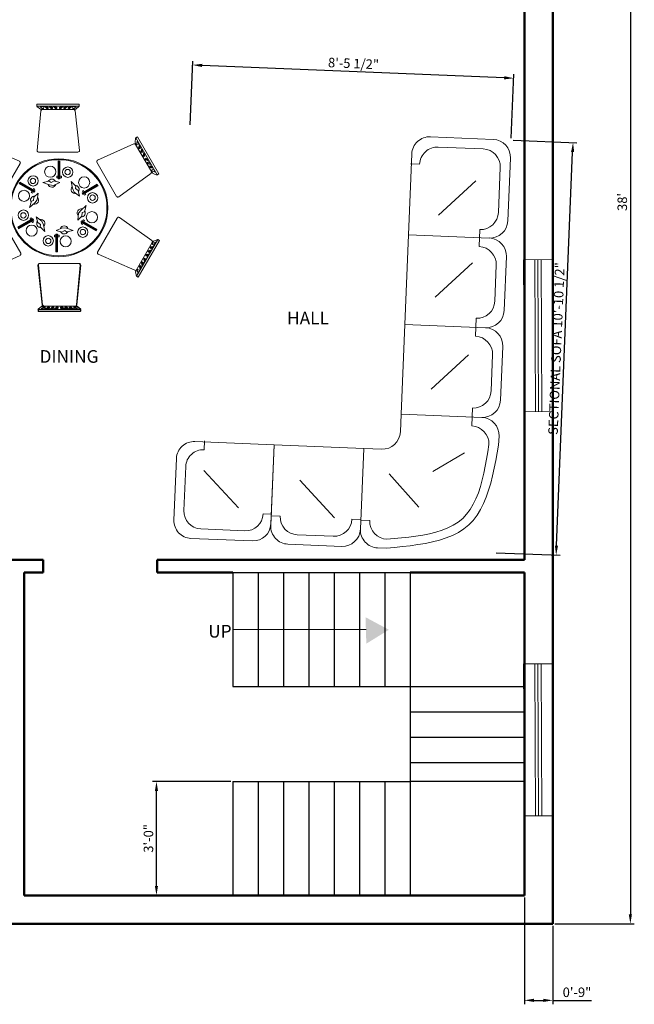
# Model space of a CAD drawing. Units: inches. Extents: x 108 to 1546, y -229 to 513.
# Tile 10 of 11: x 1352 to 1546, y -29 to 282. Entities that reach past the tile are written whole.
import ezdxf

# ---------------------------------------------------------------- set-up
doc = ezdxf.new("R2010")
doc.units = ezdxf.units.IN
for name, color, linetype, lineweight in [('A-ANNO-DIMS', 2, 'Continuous', 18), ('A-ANNO-SYMB', 4, 'Continuous', 18), ('A-AREA-IDEN', 4, 'Continuous', 18), ('A-FLOR-STRS', 7, 'Continuous', 25), ('A-FURN', 8, 'Continuous', 13), ('wall', 7, 'Continuous', 50), ('WINDOW', 212, 'Continuous', 18)]:
    doc.layers.add(name, color=color, linetype=linetype, lineweight=lineweight)
doc.styles.get("Standard").update_dxf_attribs({"font": 'arial.ttf'})
doc.dimstyles.new('ISO-25', dxfattribs={"dimtxt": 3, "dimasz": 3, "dimexe": 1.25, "dimexo": 0.625, "dimtad": 1, "dimdec": 1, "dimlunit": 3, "dimtxsty": 'Standard', "dimcen": 2.5, "dimadec": 0, "dimazin": 0, "dimtfac": 1, "dimtdec": 1, "dimtmove": 0, "dimatfit": 3, "dimfxl": 1, "dimarcsym": 0})

# ---------------------------------------------------------------- blocks, each defined once
blk = doc.blocks.new('A$C45501D90')
for p, q in [((-242, 1134), (224, 1134)), ((-242, 1113), (-242, 1134)), ((224, 1113), (-242, 1113)), ((-242, 1111), (-202, 1079)), ((-204, 1106), (-166, 1108)), ((-169, 1081), (-204, 1106)), ((-202, 1079), (-169, 1081)), ((-166, 1108), (-167, 1086)), ((-156, 1110), (-132, 1086)), ((-119, 1086), (-143, 1108)), ((-143, 1108), (-134, 1108)), ((-134, 1108), (-122, 1098)), ((-132, 1086), (-119, 1086)), ((-122, 1098), (-119, 1102)), ((-119, 1102), (-118, 1087)), ((-108, 1110), (-84, 1086)), ((-71, 1086), (-95, 1108)), ((-95, 1108), (-86, 1108)), ((-86, 1108), (-75, 1098)), ((-84, 1086), (-71, 1086)), ((-75, 1098), (-71, 1102)), ((-71, 1102), (-70, 1087)), ((-60, 1110), (-36, 1086)), ((-23, 1086), (-47, 1108)), ((-47, 1108), (-38, 1108)), ((-38, 1108), (-27, 1098)), ((-36, 1086), (-23, 1086)), ((-27, 1098), (-23, 1102)), ((-23, 1102), (-22, 1087)), ((8, 1102), (7, 1087)), ((8, 1086), (32, 1108)), ((12, 1098), (8, 1102)), ((21, 1086), (8, 1086)), ((23, 1108), (12, 1098)), ((45, 1110), (21, 1086)), ((32, 1108), (23, 1108)), ((56, 1102), (55, 1087)), ((56, 1086), (80, 1108)), ((60, 1098), (56, 1102)), ((69, 1086), (56, 1086)), ((71, 1108), (60, 1098)), ((93, 1110), (69, 1086)), ((80, 1108), (71, 1108)), ((104, 1102), (103, 1087)), ((104, 1086), (128, 1108)), ((107, 1098), (104, 1102)), ((117, 1086), (104, 1086)), ((119, 1108), (107, 1098)), ((141, 1110), (117, 1086)), ((128, 1108), (119, 1108)), ((189, 1106), (151, 1108)), ((151, 1108), (152, 1086)), ((154, 1081), (189, 1106)), ((187, 1079), (154, 1081)), ((224, 1113), (187, 1079)), ((224, 1134), (224, 1113)), ((-197, 1062), (-239, 628)), ((162, 1076), (-181, 1076)), ((225, 628), (178, 1062)), ((-1103, 357), (-870, 761)), ((-870, 761), (-852, 750)), ((841, 765), (834, 715)), ((843, 766), (861, 776)), ((1076, 362), (843, 766)), ((861, 776), (1094, 373)), ((-852, 750), (-1085, 347)), ((-851, 678), (-1023, 381)), ((-895, 665), (-900, 657)), ((-900, 657), (-898, 642)), ((-888, 633), (-895, 665)), ((-890, 677), (-882, 644)), ((-864, 717), (-884, 684)), ((-884, 684), (-864, 675)), ((-859, 674), (-864, 717)), ((-841, 702), (-859, 674)), ((-849, 752), (-841, 702)), ((-431, 509), (-831, 685)), ((821, 702), (424, 521)), ((834, 715), (852, 687)), ((1013, 398), (841, 695)), ((852, 687), (856, 730)), ((856, 730), (877, 697)), ((877, 697), (857, 688)), ((883, 690), (874, 657)), ((874, 657), (881, 646)), ((881, 646), (888, 678)), ((894, 654), (883, 646)), ((888, 678), (893, 670)), ((893, 670), (890, 655)), ((890, 655), (894, 654)), ((907, 648), (898, 616)), ((-945, 559), (-950, 558)), ((-950, 558), (-938, 550)), ((-943, 582), (-948, 574)), ((-948, 574), (-945, 559)), ((-936, 550), (-943, 582)), ((-938, 594), (-930, 561)), ((-930, 561), (-936, 550)), ((-921, 601), (-926, 600)), ((-926, 600), (-914, 591)), ((-919, 624), (-924, 615)), ((-924, 615), (-921, 601)), ((-912, 592), (-919, 624)), ((-914, 635), (-906, 603)), ((-906, 603), (-912, 592)), ((-898, 642), (-902, 641)), ((-902, 641), (-890, 633)), ((-882, 644), (-888, 633)), ((-223, 610), (209, 610)), ((898, 616), (904, 605)), ((904, 605), (912, 637)), ((918, 613), (907, 604)), ((912, 637), (917, 628)), ((917, 628), (914, 614)), ((914, 614), (918, 613)), ((931, 607), (922, 574)), ((922, 574), (928, 563)), ((928, 563), (936, 595)), ((942, 571), (931, 563)), ((936, 595), (941, 587)), ((941, 587), (938, 572)), ((938, 572), (942, 571)), ((958, 543), (945, 538)), ((957, 539), (958, 543)), ((-1000, 440), (-1031, 430)), ((-1031, 430), (-1026, 438)), ((-1026, 438), (-1012, 443)), ((-1015, 461), (-982, 470)), ((-1012, 443), (-1014, 448)), ((-1014, 448), (-1000, 442)), ((-976, 481), (-1007, 471)), ((-1007, 471), (-1002, 480)), ((-1006, 428), (-1000, 440)), ((-1002, 480), (-989, 485)), ((-991, 503), (-958, 511)), ((-989, 485), (-990, 489)), ((-990, 489), (-976, 483)), ((-952, 522), (-983, 513)), ((-983, 513), (-978, 521)), ((-982, 470), (-976, 481)), ((-978, 521), (-965, 526)), ((-965, 526), (-966, 530)), ((-966, 530), (-953, 525)), ((-958, 511), (-952, 522)), ((-640, 112), (-424, 486)), ((-6, 509, 91), (0, 509, 91)), ((-6, 318, 91), (-6, 509, 91)), ((0, 509, 91), (0, 318, 91)), ((6, 318, 91), (6, 509, 91)), ((6, 509, 91), (12, 509, 91)), ((12, 509, 91), (12, 318, 91)), ((417, 498), (633, 124)), ((951, 524), (944, 535)), ((944, 535), (976, 526)), ((983, 516), (951, 524)), ((971, 534), (957, 539)), ((968, 494), (1000, 484)), ((975, 483), (968, 494)), ((982, 502), (969, 496)), ((976, 526), (971, 534)), ((1007, 474), (975, 483)), ((981, 498), (982, 502)), ((995, 493), (981, 498)), ((999, 441), (992, 453)), ((992, 453), (1024, 443)), ((1006, 461), (993, 455)), ((1000, 484), (995, 493)), ((1031, 433), (999, 441)), ((1005, 456), (1006, 461)), ((1019, 451), (1005, 456)), ((1024, 443), (1019, 451)), ((-1085, 347), (-1103, 357)), ((-1083, 346), (-1036, 364)), ((-1060, 377), (-1042, 411)), ((-1020, 394), (-1060, 377)), ((-1042, 411), (-1024, 398)), ((-1039, 420), (-1006, 428)), ((-1036, 364), (-1020, 394)), ((-1018, 360), (-663, 107)), ((-22, 329, 91), (-22, 345, 91)), ((-22, 345, 91), (-6, 345, 91)), ((-6, 329, 91), (-22, 329, 91)), ((0, 345, 91), (6, 345, 91)), ((6, 329, 91), (0, 329, 91)), ((12, 345, 91), (27, 345, 91)), ((27, 329, 91), (12, 329, 91)), ((27, 345, 91), (27, 329, 91)), ((656, 119), (1008, 377)), ((1028, 377), (1013, 407)), ((1013, 407), (1053, 390)), ((1035, 424), (1016, 411)), ((1076, 359), (1028, 377)), ((1053, 390), (1035, 424)), ((1094, 373), (1076, 362)), ((-436, 265, 91), (-433, 271, 91)), ((-271, 170, 91), (-436, 265, 91)), ((-433, 271, 91), (-268, 175, 91)), ((-431, 275, 91), (-428, 280, 91)), ((-265, 180, 91), (-431, 275, 91)), ((-428, 280, 91), (-262, 185, 91)), ((-175, 276, 91), (-105, 293, 91)), ((-103, 252, 91), (-175, 276, 91)), ((-105, 293, 91), (-86, 278, 91)), ((-60, 246, 91), (-103, 252, 91)), ((-86, 278, 91), (-52, 294, 91)), ((9, 276, 91), (-60, 246, 91)), ((-52, 294, 91), (9, 276, 91)), ((0, 318, 91), (-6, 318, 91)), ((12, 318, 91), (6, 318, 91)), ((134, 288, 91), (184, 236, 91)), ((150, 214, 91), (134, 288, 91)), ((184, 236, 91), (181, 211, 91)), ((255, 162, 91), (421, 257, 91)), ((424, 252, 91), (258, 157, 91)), ((261, 152, 91), (426, 248, 91)), ((429, 242, 91), (264, 147, 91)), ((421, 257, 91), (424, 252, 91)), ((426, 248, 91), (429, 242, 91)), ((-303, 169, 91), (-294, 183, 91)), ((-289, 161, 91), (-303, 169, 91)), ((-291, 188, 91), (-289, 193, 91)), ((-281, 176, 91), (-289, 161, 91)), ((-286, 198, 91), (-278, 212, 91)), ((-278, 212, 91), (-264, 204, 91)), ((-275, 185, 91), (-278, 181, 91)), ((-277, 81, 91), (-274, 118, 91)), ((-274, 118, 91), (-227, 162, 91)), ((-264, 204, 91), (-272, 191, 91)), ((-268, 175, 91), (-271, 170, 91)), ((-262, 185, 91), (-265, 180, 91)), ((-227, 162, 91), (-236, 87, 91)), ((166, 173, 91), (150, 214, 91)), ((227, 128, 91), (166, 173, 91)), ((181, 211, 91), (211, 190, 91)), ((211, 190, 91), (227, 128, 91)), ((258, 157, 91), (255, 162, 91)), ((257, 182, 91), (270, 190, 91)), ((265, 168, 91), (257, 182, 91)), ((264, 147, 91), (261, 152, 91)), ((271, 158, 91), (268, 162, 91)), ((270, 190, 91), (278, 175, 91)), ((281, 139, 91), (274, 153, 91)), ((281, 170, 91), (284, 165, 91)), ((295, 147, 91), (281, 139, 91)), ((287, 160, 91), (295, 147, 91)), ((-320, 2, 91), (-299, 72, 91)), ((-263, 53, 91), (-320, 2, 91)), ((-299, 72, 91), (-277, 81, 91)), ((-236, 87, 91), (-263, 53, 91)), ((243, -25, 91), (299, 26, 91)), ((299, 26, 91), (279, -44, 91)), ((-247, -100, 91), (-187, -145, 91)), ((-232, -162, 91), (-247, -100, 91)), ((207, -134, 91), (216, -60, 91)), ((253, -90, 91), (207, -134, 91)), ((216, -60, 91), (243, -25, 91)), ((256, -53, 91), (253, -90, 91)), ((279, -44, 91), (256, -53, 91)), ((1018, -360), (663, -107)), ((-656, -119), (-1008, -377)), ((-417, -498), (-633, -124)), ((-450, -214, 91), (-284, -119, 91)), ((-447, -220, 91), (-450, -214, 91)), ((-281, -124, 91), (-447, -220, 91)), ((-444, -224, 91), (-279, -129, 91)), ((-276, -134, 91), (-441, -229, 91)), ((-315, -119, 91), (-302, -111, 91)), ((-307, -132, 91), (-315, -119, 91)), ((-302, -142, 91), (-304, -137, 91)), ((-302, -111, 91), (-294, -125, 91)), ((-290, -162, 91), (-299, -147, 91)), ((-291, -130, 91), (-288, -134, 91)), ((-277, -154, 91), (-290, -162, 91)), ((-285, -140, 91), (-277, -154, 91)), ((-284, -119, 91), (-281, -124, 91)), ((-279, -129, 91), (-276, -134, 91)), ((-201, -183, 91), (-232, -162, 91)), ((-205, -208, 91), (-201, -183, 91)), ((-155, -260, 91), (-205, -208, 91)), ((-187, -145, 91), (-170, -186, 91)), ((-170, -186, 91), (-155, -260, 91)), ((242, -157, 91), (245, -152, 91)), ((407, -252, 91), (242, -157, 91)), ((244, -176, 91), (252, -163, 91)), ((257, -184, 91), (244, -176, 91)), ((245, -152, 91), (410, -247, 91)), ((248, -147, 91), (251, -142, 91)), ((413, -243, 91), (248, -147, 91)), ((251, -142, 91), (416, -237, 91)), ((255, -157, 91), (257, -153, 91)), ((265, -170, 91), (257, -184, 91)), ((260, -148, 91), (269, -133, 91)), ((271, -160, 91), (268, -165, 91)), ((269, -133, 91), (282, -141, 91)), ((282, -141, 91), (274, -155, 91)), ((640, -112), (424, -486)), ((-441, -229, 91), (-444, -224, 91)), ((-48, -317, 91), (-48, -301, 91)), ((-48, -301, 91), (-32, -301, 91)), ((-32, -317, 91), (-48, -317, 91)), ((-32, -481, 91), (-32, -290, 91)), ((-32, -290, 91), (-26, -290, 91)), ((-30, -248, 91), (39, -218, 91)), ((32, -266, 91), (-30, -248, 91)), ((-26, -290, 91), (-26, -481, 91)), ((-26, -301, 91), (-21, -301, 91)), ((-21, -317, 91), (-26, -317, 91)), ((-21, -481, 91), (-21, -290, 91)), ((-21, -290, 91), (-15, -290, 91)), ((-15, -290, 91), (-15, -481, 91)), ((-15, -301, 91), (2, -301, 91)), ((2, -317, 91), (-15, -317, 91)), ((2, -301, 91), (2, -317, 91)), ((65, -250, 91), (32, -266, 91)), ((39, -218, 91), (83, -224, 91)), ((84, -265, 91), (65, -250, 91)), ((83, -224, 91), (155, -248, 91)), ((155, -248, 91), (84, -265, 91)), ((410, -247, 91), (407, -252, 91)), ((416, -237, 91), (413, -243, 91)), ((-1094, -373), (-1076, -362)), ((-861, -776), (-1094, -373)), ((-1076, -359), (-1028, -377)), ((-1076, -362), (-843, -766)), ((-1053, -390), (-1035, -424)), ((-1013, -407), (-1053, -390)), ((-1035, -424), (-1016, -411)), ((-1028, -377), (-1013, -407)), ((-1013, -398), (-841, -695)), ((851, -678), (1023, -381)), ((852, -750), (1085, -347)), ((1103, -357), (870, -761)), ((1006, -428), (1000, -440)), ((1000, -440), (1031, -430)), ((1039, -420), (1006, -428)), ((1036, -364), (1020, -394)), ((1020, -394), (1060, -377)), ((1042, -411), (1024, -398)), ((1031, -430), (1026, -438)), ((1083, -346), (1036, -364)), ((1060, -377), (1042, -411)), ((1085, -347), (1103, -357)), ((-1031, -433), (-999, -441)), ((-1024, -443), (-1019, -451)), ((-992, -453), (-1024, -443)), ((-1019, -451), (-1005, -456)), ((-1007, -474), (-975, -483)), ((-1006, -461), (-993, -455)), ((-1005, -456), (-1006, -461)), ((-968, -494), (-1000, -484)), ((-1000, -484), (-995, -493)), ((-999, -441), (-992, -453)), ((-995, -493), (-981, -498)), ((-983, -516), (-951, -524)), ((-982, -502), (-969, -496)), ((-981, -498), (-982, -502)), ((-944, -535), (-976, -526)), ((-976, -526), (-971, -534)), ((-975, -483), (-968, -494)), ((-971, -534), (-957, -539)), ((-958, -543), (-945, -538)), ((-957, -539), (-958, -543)), ((-951, -524), (-944, -535)), ((-821, -702), (-424, -521)), ((-26, -481, 91), (-32, -481, 91)), ((-15, -481, 91), (-21, -481, 91)), ((431, -509), (831, -685)), ((958, -511), (952, -522)), ((952, -522), (983, -513)), ((966, -530), (953, -525)), ((991, -503), (958, -511)), ((978, -521), (965, -526)), ((965, -526), (966, -530)), ((982, -470), (976, -481)), ((976, -481), (1007, -471)), ((990, -489), (976, -483)), ((983, -513), (978, -521)), ((1015, -461), (982, -470)), ((1002, -480), (989, -485)), ((989, -485), (990, -489)), ((1014, -448), (1000, -442)), ((1007, -471), (1002, -480)), ((1026, -438), (1012, -443)), ((1012, -443), (1014, -448)), ((-942, -571), (-931, -563)), ((-938, -572), (-942, -571)), ((-941, -587), (-938, -572)), ((-936, -595), (-941, -587)), ((-928, -563), (-936, -595)), ((-931, -607), (-922, -574)), ((-922, -574), (-928, -563)), ((-918, -613), (-907, -604)), ((-914, -614), (-918, -613)), ((-917, -628), (-914, -614)), ((-912, -637), (-917, -628)), ((-904, -605), (-912, -637)), ((-907, -648), (-898, -616)), ((-898, -616), (-904, -605)), ((-894, -654), (-883, -646)), ((-881, -646), (-888, -678)), ((-874, -657), (-881, -646)), ((-229, -629), (-182, -1063)), ((-225, -628), (-178, -1062)), ((219, -612), (-213, -612)), ((223, -610), (-209, -610)), ((193, -1063), (235, -629)), ((197, -1062), (239, -628)), ((882, -644), (888, -633)), ((890, -677), (882, -644)), ((888, -633), (895, -665)), ((902, -641), (890, -633)), ((898, -642), (902, -641)), ((900, -657), (898, -642)), ((906, -603), (912, -592)), ((914, -635), (906, -603)), ((912, -592), (919, -624)), ((926, -600), (914, -591)), ((919, -624), (924, -615)), ((921, -601), (926, -600)), ((924, -615), (921, -601)), ((930, -561), (936, -550)), ((938, -594), (930, -561)), ((936, -550), (943, -582)), ((950, -558), (938, -550)), ((943, -582), (948, -574)), ((945, -559), (950, -558)), ((948, -574), (945, -559)), ((-890, -655), (-894, -654)), ((-893, -670), (-890, -655)), ((-888, -678), (-893, -670)), ((-883, -690), (-874, -657)), ((-877, -697), (-857, -688)), ((-856, -730), (-877, -697)), ((-852, -687), (-856, -730)), ((-834, -715), (-852, -687)), ((-841, -765), (-834, -715)), ((841, -702), (859, -674)), ((849, -752), (841, -702)), ((870, -761), (852, -750)), ((859, -674), (864, -717)), ((884, -684), (864, -675)), ((864, -717), (884, -684)), ((895, -665), (900, -657)), ((-843, -766), (-861, -776)), ((-166, -1078), (177, -1078)), ((-162, -1076), (181, -1076)), ((-231, -1113), (-191, -1081)), ((-228, -1114), (238, -1114)), ((-228, -1135), (-228, -1114)), ((238, -1135), (-228, -1135)), ((-227, -1111), (-187, -1079)), ((-224, -1113), (242, -1113)), ((-224, -1134), (-224, -1113)), ((242, -1134), (-224, -1134)), ((-158, -1082), (-193, -1108)), ((-193, -1108), (-155, -1109)), ((-191, -1081), (-158, -1082)), ((-154, -1081), (-189, -1106)), ((-189, -1106), (-151, -1108)), ((-187, -1079), (-154, -1081)), ((-155, -1109), (-156, -1087)), ((-151, -1108), (-152, -1086)), ((-145, -1111), (-121, -1087)), ((-141, -1110), (-117, -1086)), ((-108, -1087), (-132, -1109)), ((-132, -1109), (-123, -1109)), ((-104, -1086), (-128, -1108)), ((-128, -1108), (-119, -1108)), ((-123, -1109), (-112, -1100)), ((-121, -1087), (-108, -1087)), ((-119, -1108), (-107, -1098)), ((-117, -1086), (-104, -1086)), ((-112, -1100), (-108, -1103)), ((-108, -1103), (-107, -1089)), ((-107, -1098), (-104, -1102)), ((-104, -1102), (-103, -1087)), ((-97, -1111), (-73, -1087)), ((-93, -1110), (-69, -1086)), ((-60, -1087), (-84, -1109)), ((-84, -1109), (-75, -1109)), ((-56, -1086), (-80, -1108)), ((-80, -1108), (-71, -1108)), ((-75, -1109), (-64, -1100)), ((-73, -1087), (-60, -1087)), ((-71, -1108), (-60, -1098)), ((-69, -1086), (-56, -1086)), ((-64, -1100), (-60, -1103)), ((-60, -1103), (-59, -1089)), ((-60, -1098), (-56, -1102)), ((-56, -1102), (-55, -1087)), ((-49, -1111), (-25, -1087)), ((-45, -1110), (-21, -1086)), ((-13, -1087), (-37, -1109)), ((-37, -1109), (-27, -1109)), ((-8, -1086), (-32, -1108)), ((-32, -1108), (-23, -1108)), ((-27, -1109), (-16, -1100)), ((-25, -1087), (-13, -1087)), ((-23, -1108), (-12, -1098)), ((-21, -1086), (-8, -1086)), ((-16, -1100), (-13, -1103)), ((-13, -1103), (-11, -1089)), ((-12, -1098), (-8, -1102)), ((-8, -1102), (-7, -1087)), ((19, -1103), (18, -1089)), ((19, -1087), (43, -1109)), ((32, -1087), (19, -1087)), ((23, -1100), (19, -1103)), ((23, -1102), (22, -1087)), ((23, -1086), (47, -1108)), ((36, -1086), (23, -1086)), ((27, -1098), (23, -1102)), ((34, -1109), (23, -1100)), ((38, -1108), (27, -1098)), ((56, -1111), (32, -1087)), ((43, -1109), (34, -1109)), ((60, -1110), (36, -1086)), ((47, -1108), (38, -1108)), ((67, -1103), (66, -1089)), ((67, -1087), (91, -1109)), ((80, -1087), (67, -1087)), ((70, -1100), (67, -1103)), ((71, -1102), (70, -1087)), ((82, -1109), (70, -1100)), ((71, -1086), (95, -1108)), ((84, -1086), (71, -1086)), ((75, -1098), (71, -1102)), ((86, -1108), (75, -1098)), ((104, -1111), (80, -1087)), ((91, -1109), (82, -1109)), ((108, -1110), (84, -1086)), ((95, -1108), (86, -1108)), ((115, -1103), (114, -1089)), ((115, -1087), (139, -1109)), ((128, -1087), (115, -1087)), ((118, -1100), (115, -1103)), ((119, -1102), (118, -1087)), ((130, -1109), (118, -1100)), ((119, -1086), (143, -1108)), ((132, -1086), (119, -1086)), ((122, -1098), (119, -1102)), ((134, -1108), (122, -1098)), ((152, -1111), (128, -1087)), ((139, -1109), (130, -1109)), ((156, -1110), (132, -1086)), ((143, -1108), (134, -1108)), ((161, -1109), (163, -1087)), ((200, -1108), (161, -1109)), ((198, -1081), (165, -1082)), ((165, -1082), (200, -1108)), ((166, -1108), (167, -1086)), ((204, -1106), (166, -1108)), ((202, -1079), (169, -1081)), ((169, -1081), (204, -1106)), ((238, -1113), (198, -1081)), ((242, -1111), (202, -1079)), ((238, -1114), (238, -1135)), ((242, -1113), (242, -1134))]:
    blk.add_line(p, q)
for centre, radius in [((0, 0), 537), ((0, 0), 527), ((-95, 395, 91), 61.3), ((97, 390, 91), 56.9), ((-282, 295, 91), 56.9), ((96, 391, 91), 29.4), ((277, 278, 91), 61.3), ((-284, 294, 91), 29.4), ((-382, 131, 91), 61.3), ((369, 109, 91), 56.9), ((369, 111, 91), 29.4), ((-389, -81, 91), 56.9), ((-389, -83, 91), 29.4), ((362, -103, 91), 61.3), ((-298, -250, 91), 61.3), ((262, -267, 91), 56.9), ((-117, -362, 91), 56.9), ((74, -367, 91), 61.3), ((263, -266, 91), 29.4), ((-116, -363, 91), 29.4)]:
    blk.add_circle(centre, radius)
for centre, radius, start, end in [((-181, 1060), 16, 90, 174.5199), ((162, 1060), 16, 6.2572, 90), ((-837, 670), 16, 66.2572, 150), ((827, 687), 16, 30, 114.5199), ((-223, 626), 16, 174.5199, 270), ((209, 626), 16, 270, 6.2572), ((-438, 494), 16, 330, 66.2572), ((431, 506), 16, 114.5199, 210), ((-1009, 373), 16, 150, 234.5199), ((999, 390), 16, 306.2572, 30), ((-77, 270, 91), 44.6, 195.9338, 342.9389), ((-77, 270, 91), 44.6, 25.8558, 153.3359), ((178, 200, 91), 44.6, 135.9338, 282.9389), ((178, 200, 91), 44.6, 325.8558, 93.3359), ((-654, 120), 16, 234.5199, 330), ((-266, 84, 91), 44.6, 85.8558, 213.3359), ((-266, 84, 91), 44.6, 255.9338, 42.9389), ((647, 132), 16, 210, 306.2572), ((245, -56, 91), 44.6, 75.9338, 222.9389), ((245, -56, 91), 44.6, 265.8558, 33.3359), ((654, -120), 16, 54.5199, 150), ((-647, -132), 16, 30, 126.2572), ((-198, -172, 91), 44.6, 145.8558, 273.3359), ((-198, -172, 91), 44.6, 315.9338, 102.9389), ((57, -242, 91), 44.6, 15.9338, 162.9389), ((57, -242, 91), 44.6, 205.8558, 333.3359), ((-999, -390), 16, 126.2572, 210), ((1009, -373), 16, 330, 54.5199), ((-431, -506), 16, 294.5199, 30), ((438, -494), 16, 150, 246.2572), ((-213, -628), 16, 90, 186.2572), ((-209, -626), 16, 90, 186.2572), ((219, -628), 16, 354.5199, 90), ((223, -626), 16, 354.5199, 90), ((-827, -687), 16, 210, 294.5199), ((837, -670), 16, 246.2572, 330), ((-166, -1062), 16, 186.2572, 270), ((-162, -1060), 16, 186.2572, 270), ((177, -1062), 16, 270, 354.5199), ((181, -1060), 16, 270, 354.5199)]:
    blk.add_arc(centre, radius, start, end)
blk = doc.blocks.new('A$C4B324E0D')
for points in [[(-0.4032, -0.0374), (-0.3959, 0.0153), (-0.3883, 0.0678), (-0.3801, 0.1195), (-0.3709, 0.1704), (-0.3605, 0.22), (-0.3485, 0.2679), (-0.3346, 0.314), (-0.3185, 0.3579), (-0.2998, 0.3993), (-0.2783, 0.4378), (-0.2537, 0.4731), (-0.2255, 0.5049), (-0.1936, 0.5331), (-0.1583, 0.5578), (-0.1198, 0.5793), (-0.0785, 0.5979), (-0.0346, 0.614), (0.0115, 0.628), (0.0595, 0.64), (0.1091, 0.6504), (0.1599, 0.6595), (0.2117, 0.6678), (0.2641, 0.6753), (0.3168, 0.6826)], [(0.3768, 0.6826), (0.3168, 0.6826)], [(0.9768, 0.6826), (0.6168, 0.6826)], [(1.5769, 0.6826), (1.2168, 0.6826)], [(1.8168, 0.6826), (2.2368, 0.6826)], [(-0.3432, -0.0374), (-0.3369, 0.0114), (-0.3303, 0.0599), (-0.3232, 0.1078), (-0.3151, 0.1548), (-0.3059, 0.2006), (-0.2951, 0.2449), (-0.2826, 0.2874), (-0.2681, 0.3278), (-0.2511, 0.3658), (-0.2315, 0.4011), (-0.2089, 0.4335), (-0.1831, 0.4625), (-0.1538, 0.488), (-0.1214, 0.5102), (-0.086, 0.5294), (-0.0479, 0.546), (-0.0075, 0.5602), (0.035, 0.5722), (0.0793, 0.5825), (0.125, 0.5914), (0.172, 0.599), (0.2198, 0.6057), (0.2682, 0.6119), (0.3168, 0.6177)], [(0.3168, 0.6177), (0.3168, 0.6177)], [(0.9168, 0.6177), (0.6768, 0.6177)], [(1.5168, 0.6177), (1.2768, 0.6177)], [(2.1704, 0.6177), (1.8704, 0.6177)], [(0.4968, 0.0226), (0.4968, 0.5626)], [(0.4968, 0.5626), (0.4968, 0.0226), (1.0968, 0.0226)], [(1.0968, 0.5626), (1.0968, 0.0226), (1.6968, 0.0226)], [(1.0968, 0.0226), (1.0968, 0.5626)], [(1.6968, 0.0226), (1.6968, 0.5626)], [(2.2368, 0.0226), (1.6968, 0.0226), (1.6968, 0.5626)], [(2.3569, 0.5626), (2.3569, 0.1426)], [(0.4968, 0.4977), (0.4368, 0.4977), (0.4368, 0.4977)], [(0.5569, 0.4977), (0.5569, 0.4977), (0.4968, 0.4977)], [(1.0968, 0.4977), (1.0368, 0.4977), (1.0368, 0.4977)], [(1.1569, 0.4977), (1.1569, 0.4977), (1.0968, 0.4977)], [(1.6969, 0.4977), (1.6368, 0.4977), (1.6368, 0.4977)], [(1.7504, 0.4977), (1.7504, 0.4977), (1.6904, 0.4977)], [(2.2904, 0.1977), (2.2904, 0.4977)], [(0.255, 0.4573), (0.1211, 0.2495)], [(0.9111, 0.4573), (0.6711, 0.2173)], [(1.527, 0.4573), (1.287, 0.2173)], [(2.0759, 0.4573), (1.8359, 0.2173)], [(-0.1199, 0.1664), (0.0943, -0.0414)], [(2.1704, 0.0177), (2.1704, 0.0777), (2.1704, 0.0777)], [(0.4968, 0.0226), (0.3768, 0.0226)], [(-0.4032, -0.0974), (-0.4032, -0.0374)], [(-0.3432, -0.0374), (-0.3432, -0.0374)], [(0.2568, -0.0974), (0.2568, -0.2174)], [(-0.2232, -0.2174), (-0.2232, -0.1574), (-0.2232, -0.1574)], [(-0.2832, -0.8174), (0.2568, -0.8174), (0.2568, -0.2174)], [(0.2568, -0.2174), (-0.2832, -0.2174)], [(0.2568, -0.2174), (-0.2832, -0.2174)], [(-0.2183, -0.2174), (-0.2183, -0.2774), (-0.2183, -0.2774)], [(-0.4032, -0.3374), (-0.4032, -0.6974)], [(-0.2136, -0.3946), (0.0264, -0.6346)], [(-0.3383, -0.3974), (-0.3383, -0.6374)], [(-0.2183, -0.7574), (-0.2183, -0.7574), (-0.2183, -0.8174)], [(0.2568, -0.8174), (-0.2832, -0.8174)], [(-0.2732, -0.8174), (0.2568, -0.8174), (0.2568, -1.3475)], [(-0.208, -0.8126), (-0.208, -0.8715), (-0.208, -0.8715)], [(0.2568, -0.8174), (0.2568, -1.3475)], [(-0.391, -1.3475), (-0.391, -0.9352)], [(-0.3258, -0.9893), (-0.3258, -1.2838)], [(-0.1734, -1.0387), (0.0666, -1.2787)], [(0.2043, -1.2838), (0.2043, -1.2838), (0.2632, -1.2838)], [(-0.208, -1.4016), (0.0865, -1.4016)], [(0.1391, -1.4653), (-0.2732, -1.4653)]]:
    blk.add_lwpolyline(points)
for centre, radius, start, end in [((0.3768, 0.5626), 0.12, 0, 90), ((0.6168, 0.5626), 0.12, 90, 180), ((0.9768, 0.5626), 0.12, 0, 90), ((1.2168, 0.5626), 0.12, 90, 180), ((1.5769, 0.5626), 0.12, 0, 90), ((1.8168, 0.5626), 0.12, 90, 180), ((2.2368, 0.5626), 0.12, 0, 90), ((0.3168, 0.4977), 0.12, 0, 90), ((0.6768, 0.4977), 0.12, 90, 180), ((0.9168, 0.4977), 0.12, 0, 90), ((1.2768, 0.4977), 0.12, 90, 180), ((1.5168, 0.4977), 0.12, 0, 90), ((1.8704, 0.4977), 0.12, 90, 180), ((2.1704, 0.4977), 0.12, 0, 90), ((2.1704, 0.1977), 0.12, 270, 0), ((2.2368, 0.1426), 0.12, 270, 0), ((0.3768, -0.0974), 0.12, 90, 180), ((-0.2232, -0.0374), 0.12, 180, 270), ((-0.2832, -0.0974), 0.12, 179.9997, 270), ((-0.2832, -0.3374), 0.12, 90, 180), ((-0.2183, -0.3974), 0.12, 90, 180), ((-0.2183, -0.6374), 0.12, 180, 270), ((-0.2832, -0.6974), 0.12, 179.9997, 270), ((-0.2732, -0.9352), 0.1178, 90, 180), ((-0.208, -0.9893), 0.1178, 90, 180), ((-0.208, -1.2838), 0.1178, 180, 270), ((0.0865, -1.2838), 0.1178, 270, 0), ((-0.2732, -1.3475), 0.1178, 179.9997, 270), ((0.1391, -1.3475), 0.1178, 270, 0)]:
    blk.add_arc(centre, radius, start, end)
blk = doc.blocks.new('A$C58C6152E')
at = {"xscale": 1.5, "yscale": 1.5, "zscale": 1.5, "rotation": 90}
blk.add_blockref('A$C4B324E0D', (1.0239, 0.6047), dxfattribs=at)
blk = doc.blocks.new('A$C15DC316E')
at = {"xscale": -1, "rotation": 270}
blk.add_blockref('A$C58C6152E', (0, 0), dxfattribs=at)
blk = doc.blocks.new('*D26')
at = {"layer": 'A-ANNO-DIMS', "color": 0, "lineweight": -2, "transparency": 16777216}
for p, q in [((1520.57, 452.47), (1545.65, 452.47)), ((1544.4, 449.47), (1544.4, -0.53)), ((1520.57, -3.53), (1545.65, -3.53))]:
    blk.add_line(p, q, dxfattribs=at)
at = {"layer": 'A-ANNO-DIMS', "color": 0, "transparency": 16777216}
for points in [[(1543.9, 449.47), (1544.9, 449.47), (1544.4, 452.47)], [(1543.9, -0.53), (1544.9, -0.53), (1544.4, -3.53)]]:
    blk.add_solid(points, dxfattribs=at)
at = {"layer": 'Defpoints', "color": 0, "transparency": 16777216}
for p in [(1519.94, 452.47), (1519.94, -3.53), (1544.4, -3.53)]:
    blk.add_point(p, dxfattribs=at)
at = {"layer": 'A-ANNO-DIMS', "color": 0, "transparency": 16777216, "insert": (1542.24, 224.47), "char_height": 3, "attachment_point": 5, "rotation": 90}
blk.add_mtext("38'", dxfattribs=at)
blk = doc.blocks.new('WINDOW-48X9')
for p, q in [((0, 9), (0, 0)), ((0, 9), (48, 9)), ((48, 9), (48, 0)), ((0, 5.5), (48, 5.5)), ((0, 4.5), (48, 4.5)), ((0, 3.5), (48, 3.5)), ((0, 0), (48, 0))]:
    blk.add_line(p, q)
blk = doc.blocks.new('*D70')
at = {"layer": 'A-ANNO-DIMS', "color": 0, "lineweight": -2, "transparency": 16777216}
for p, q in [((1507.38, 243.98), (1527.54, 243.16)), ((1521.07, 115.92), (1526.17, 240.21)), ((1502.03, 113.7), (1522.2, 112.87))]:
    blk.add_line(p, q, dxfattribs=at)
at = {"layer": 'A-ANNO-DIMS', "color": 0, "transparency": 16777216}
for points in [[(1525.67, 240.23), (1526.67, 240.19), (1526.3, 243.21)], [(1520.57, 115.94), (1521.57, 115.9), (1520.95, 112.92)]]:
    blk.add_solid(points, dxfattribs=at)
at = {"layer": 'Defpoints', "color": 0, "transparency": 16777216}
for p in [(1506.75, 244.01), (1526.3, 243.21), (1501.41, 113.72)]:
    blk.add_point(p, dxfattribs=at)
at = {"layer": 'A-ANNO-DIMS', "color": 0, "transparency": 16777216, "insert": (1521.45, 178.15), "char_height": 3, "attachment_point": 5, "rotation": 87.6494}
blk.add_mtext('SECTIONAL SOFA 10\'-10 1/2"', dxfattribs=at)
blk = doc.blocks.new('*D71')
at = {"layer": 'A-ANNO-DIMS', "color": 0, "lineweight": -2, "transparency": 16777216}
for p, q in [((1405.39, 248.79), (1406.22, 268.96)), ((1504.56, 263.67), (1409.17, 267.59)), ((1506.78, 244.63), (1507.61, 264.8))]:
    blk.add_line(p, q, dxfattribs=at)
at = {"layer": 'A-ANNO-DIMS', "color": 0, "transparency": 16777216}
for points in [[(1409.19, 268.09), (1409.14, 267.09), (1406.17, 267.71)], [(1504.58, 264.17), (1504.54, 263.17), (1507.56, 263.55)]]:
    blk.add_solid(points, dxfattribs=at)
at = {"layer": 'Defpoints', "color": 0, "transparency": 16777216}
for p in [(1406.17, 267.71), (1405.37, 248.17), (1506.75, 244.01)]:
    blk.add_point(p, dxfattribs=at)
at = {"layer": 'A-ANNO-DIMS', "color": 0, "transparency": 16777216, "insert": (1456.95, 267.81), "char_height": 3, "attachment_point": 5, "rotation": 357.6494}
blk.add_mtext('8\'-5 1/2"', dxfattribs=at)
blk = doc.blocks.new('*D109')
at = {"layer": 'A-ANNO-DIMS', "color": 0, "lineweight": -2, "transparency": 16777216}
for p, q in [((1418.27, 41.47), (1393.49, 41.47)), ((1394.74, 8.47), (1394.74, 38.47)), ((1418.27, 5.47), (1393.49, 5.47))]:
    blk.add_line(p, q, dxfattribs=at)
at = {"layer": 'A-ANNO-DIMS', "color": 0, "transparency": 16777216}
for points in [[(1394.24, 38.47), (1395.24, 38.47), (1394.74, 41.47)], [(1394.24, 8.47), (1395.24, 8.47), (1394.74, 5.47)]]:
    blk.add_solid(points, dxfattribs=at)
at = {"layer": 'Defpoints', "color": 0, "transparency": 16777216}
for p in [(1394.74, 41.47), (1418.89, 41.47), (1418.89, 5.47)]:
    blk.add_point(p, dxfattribs=at)
at = {"layer": 'A-ANNO-DIMS', "color": 0, "transparency": 16777216, "insert": (1392.59, 23.47), "char_height": 3, "attachment_point": 5, "rotation": 90}
blk.add_mtext('3\'-0"', dxfattribs=at)
blk = doc.blocks.new('*D110')
at = {"layer": 'A-ANNO-DIMS', "color": 0, "lineweight": -2, "transparency": 16777216}
for p, q in [((1510.94, 4.84), (1510.94, -28.93)), ((1519.94, -4.16), (1519.94, -28.93)), ((1513.94, -27.68), (1516.94, -27.68)), ((1519.94, -27.68), (1532.16, -27.68))]:
    blk.add_line(p, q, dxfattribs=at)
at = {"layer": 'A-ANNO-DIMS', "color": 0, "transparency": 16777216}
for points in [[(1513.94, -27.18), (1513.94, -28.18), (1510.94, -27.68)], [(1516.94, -27.18), (1516.94, -28.18), (1519.94, -27.68)]]:
    blk.add_solid(points, dxfattribs=at)
at = {"layer": 'Defpoints', "color": 0, "transparency": 16777216}
for p in [(1510.94, 5.47), (1519.94, -3.53), (1519.94, -27.68)]:
    blk.add_point(p, dxfattribs=at)
at = {"layer": 'A-ANNO-DIMS', "color": 0, "transparency": 16777216, "insert": (1527.55, -25.52), "char_height": 3, "attachment_point": 5}
blk.add_mtext('0\'-9"', dxfattribs=at)

msp = doc.modelspace()

# ---------------------------------------------------------------- hatches: boundary and pattern name
at = {"layer": 'A-ANNO-SYMB'}
h = msp.add_hatch(color=256, dxfattribs=at)
h.dxf.hatch_style = 1
h.paths.add_polyline_path([(1461.02, 84.96), (1468.13, 89.36), (1465.28, 90.89), (1460.91, 88.47)])
h.paths.add_polyline_path([(1460.91, 88.47), (1465.28, 90.89), (1460.76, 93.32)])

# ---------------------------------------------------------------- linework, layer by layer
msp.add_line((1418.89, 89.47), (1460.99, 89.47), dxfattribs=at)
at = {"layer": 'A-FLOR-STRS'}
for p, q in [((1418.89, 107.47), (1418.89, 71.47)), ((1418.89, 107.47), (1474.89, 107.47)), ((1426.89, 107.47), (1426.89, 71.47)), ((1434.89, 107.47), (1434.89, 71.47)), ((1442.89, 107.47), (1442.89, 71.47)), ((1450.89, 107.47), (1450.89, 71.47)), ((1458.89, 107.47), (1458.89, 71.47)), ((1466.89, 107.47), (1466.89, 71.47)), ((1510.89, 107.47), (1474.89, 107.47)), ((1474.89, 107.47), (1474.89, 71.47)), ((1510.89, 71.47), (1510.89, 107.47)), ((1418.89, 71.47), (1474.89, 71.47)), ((1474.89, 71.47), (1510.89, 71.47)), ((1474.89, 71.47), (1474.89, 41.47)), ((1474.89, 63.47), (1510.89, 63.47)), ((1474.89, 55.47), (1510.89, 55.47)), ((1474.89, 47.47), (1510.89, 47.47)), ((1418.89, 41.47), (1418.89, 5.47)), ((1418.89, 41.47), (1474.89, 41.47)), ((1426.89, 41.47), (1426.89, 5.47)), ((1434.89, 41.47), (1434.89, 5.47)), ((1442.89, 41.47), (1442.89, 5.47)), ((1450.89, 41.47), (1450.89, 5.47)), ((1458.89, 41.47), (1458.89, 5.47)), ((1466.89, 41.47), (1466.89, 5.47)), ((1474.89, 41.47), (1474.89, 5.47)), ((1510.89, 41.47), (1474.89, 41.47)), ((1474.89, 41.47), (1474.89, 5.47)), ((1510.89, 5.47), (1510.89, 41.47)), ((1418.89, 5.47), (1474.89, 5.47)), ((1474.89, 5.47), (1510.89, 5.47))]:
    msp.add_line(p, q, dxfattribs=at)
at = {"layer": 'wall'}
for p, q in [((1519.94, -3.53), (1519.94, 452.47)), ((1510.94, 111.47), (1510.94, 295.47)), ((1358.94, 111.47), (1343.06, 111.47)), ((1358.94, 107.47), (1358.94, 111.47)), ((1510.94, 111.47), (1394.94, 111.47)), ((1394.94, 107.47), (1394.94, 111.47)), ((1352.94, 107.47), (1352.94, 5.47)), ((1358.94, 107.47), (1352.94, 107.47)), ((1418.89, 107.47), (1394.94, 107.47)), ((1510.94, 107.47), (1474.89, 107.47)), ((1510.94, 5.47), (1510.94, 107.47)), ((1352.94, 5.47), (1510.94, 5.47)), ((1195.94, -3.53), (1519.94, -3.53))]:
    msp.add_line(p, q, dxfattribs=at)

# ---------------------------------------------------------------- block references
at = {"layer": 'A-FURN', "xscale": 0.0288298030706011, "yscale": 0.0288298030706011, "zscale": 0.0288298030706011}
msp.add_blockref('A$C45501D90', (1363.92, 222.62, -2.62), dxfattribs=at)
at = {"layer": 'A-FURN', "xscale": 31.49606299212599, "yscale": 31.49606299212599, "zscale": 31.49606299212599, "rotation": 87.64939687796358}
msp.add_blockref('A$C15DC316E', (1501.41, 113.72), dxfattribs=at)
at = {"layer": 'WINDOW'}
for p, rotation in [((1519.94, 158.24), 90.27995600981023), ((1519.94, 30.6), 90.27995600980915)]:
    msp.add_blockref('WINDOW-48X9', p, dxfattribs=dict(at, rotation=rotation))

# ---------------------------------------------------------------- texts
at = {"layer": 'A-ANNO-SYMB', "insert": (1411.09, 90.88), "char_height": 4, "attachment_point": 1}
msp.add_mtext_dynamic_manual_height_columns('UP', width=57.4311, gutter_width=12.5, heights=[12.84], dxfattribs=at)
at = {"layer": 'A-AREA-IDEN', "char_height": 4, "attachment_point": 1}
for s, insert in [('HALL', (1435.99, 189.77)), ('DINING', (1357.83, 177.67))]:
    msp.add_mtext_dynamic_manual_height_columns(s, width=57.4311, gutter_width=12.5, heights=[12.84], dxfattribs=dict(at, insert=insert))

# ---------------------------------------------------------------- dimensions: what is measured, and where the dimension line sits
at = {"layer": 'A-ANNO-DIMS'}
for base, p1, p2, angle, override, picture, middle in [((1544.4, -3.53), (1519.94, 452.47), (1519.94, -3.53), 90, {"dimclrd": 0, "dimclre": 0, "dimclrt": 0}, '*D26', (1542.24, 224.47)), ((1406.17, 267.71), (1506.75, 244.01), (1405.37, 248.17), 177.6494, {"dimdec": 1, "dimlfac": 1, "dimrnd": 0, "dimzin": 1, "dimdsep": 46, "dimlunit": 4, "dimfrac": 2}, '*D71', (1456.95, 267.81)), ((1394.74, 41.47), (1418.89, 5.47), (1418.89, 41.47), 90, {"dimdec": 1, "dimlfac": 1, "dimrnd": 0, "dimzin": 1, "dimdsep": 46, "dimlunit": 4, "dimfrac": 2}, '*D109', (1392.59, 23.47))]:
    dim = msp.add_linear_dim(base=base, p1=p1, p2=p2, angle=angle, dimstyle='ISO-25', override=override, dxfattribs=at)
    dim.commit()
    dim.dimension.update_dxf_attribs({"geometry": picture, "text_midpoint": middle})
dim = msp.add_linear_dim(base=(1526.3, 243.21), p1=(1501.41, 113.72), p2=(1506.75, 244.01), angle=87.6494, text='SECTIONAL SOFA <>', dimstyle='ISO-25', override={"dimdec": 1, "dimlfac": 1, "dimrnd": 0, "dimzin": 1, "dimdsep": 46, "dimlunit": 4, "dimfrac": 2}, dxfattribs=at)
dim.commit()
dim.dimension.update_dxf_attribs({"geometry": '*D70', "text_midpoint": (1521.45, 178.15)})
dim = msp.add_linear_dim(base=(1519.94, -27.68), p1=(1510.94, 5.47), p2=(1519.94, -3.53), dimstyle='ISO-25', override={"dimdec": 1, "dimlfac": 1, "dimrnd": 0, "dimzin": 1, "dimdsep": 46, "dimlunit": 4, "dimfrac": 2}, dxfattribs=at)
dim.commit()
dim.dimension.update_dxf_attribs({"geometry": '*D110', "text_midpoint": (1527.55, -25.52)})

doc.saveas('drawing.dxf')
